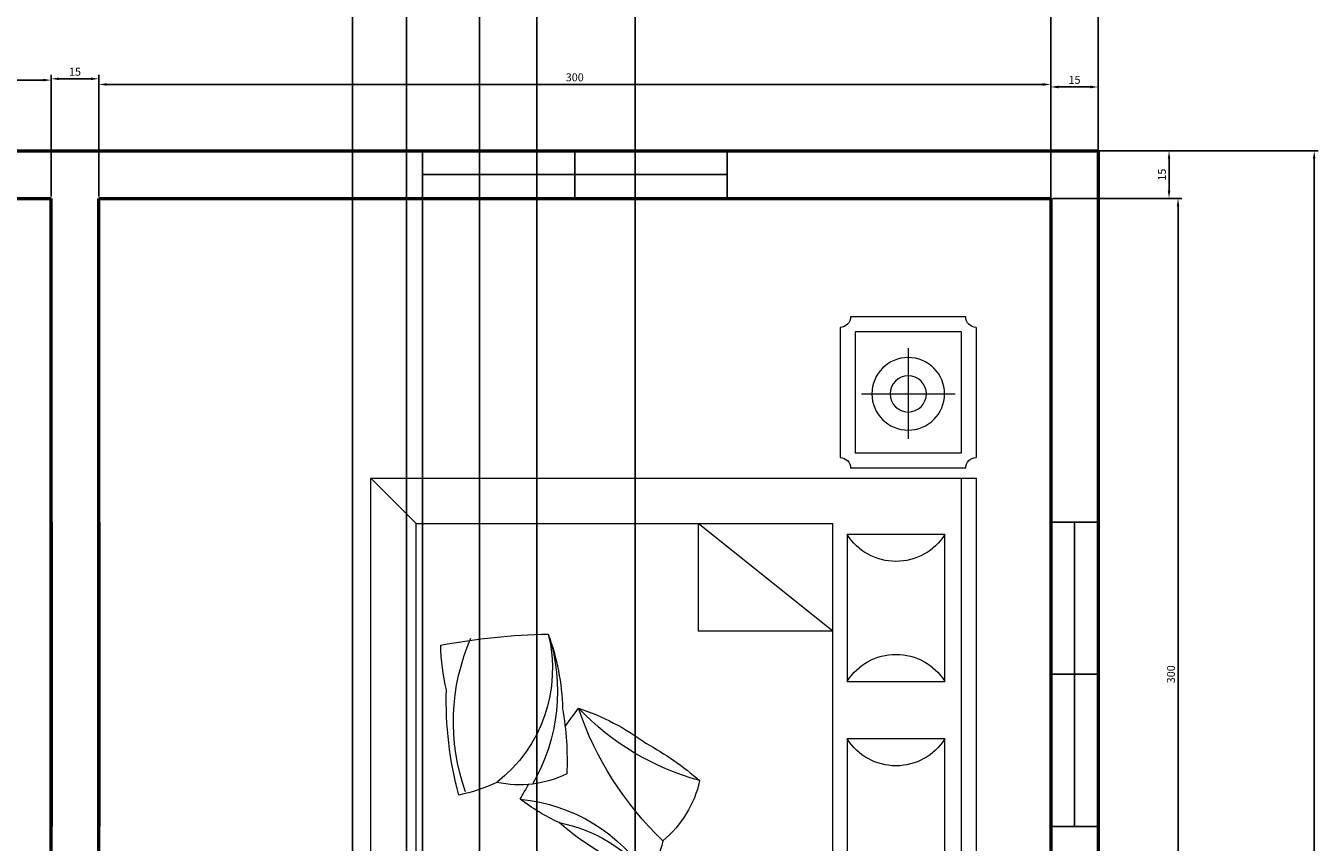
# Model space of a CAD drawing. Units: inches. Extents: x 604 to 3492, y -123 to 1737.
# Tile 17 of 20: x 1912 to 2319, y 1070 to 1327. Entities that reach past the tile are written whole.
import ezdxf

# ---------------------------------------------------------------- set-up
doc = ezdxf.new("R2010")
doc.units = ezdxf.units.IN
for name, color, linetype, lineweight in [('A-ANNO-DIMS', 2, 'Continuous', 18), ('A-FURN', 8, 'Continuous', 18), ('A-GLAZ', 4, 'Continuous', 25), ('A-WALL', 7, 'Continuous', 50)]:
    doc.layers.add(name, color=color, linetype=linetype, lineweight=lineweight)
doc.styles.get("Standard").update_dxf_attribs({"font": 'arial.ttf'})
doc.dimstyles.new('ISO-25', dxfattribs={"dimtxt": 2.5, "dimasz": 2.5, "dimexe": 1.25, "dimexo": 0.625, "dimtad": 1, "dimtxsty": 'Standard', "dimcen": 2.5, "dimadec": 0, "dimazin": 0, "dimtfac": 1, "dimtmove": 0, "dimatfit": 3, "dimfxl": 1, "dimarcsym": 0})

# ---------------------------------------------------------------- blocks, each defined once
blk = doc.blocks.new('A$C50B66110')
for p, q in [((0.0503, 1.9981), (0.4803, 1.9981)), ((0.1513, 1.6871), (0.1513, 1.9967)), ((0.5716, 1.9488), (0.5716, 2)), ((0.5716, 2), (2.0719, 2)), ((2.0719, 1.9488), (2.0719, 2)), ((2.1051, 1.9643), (2.1051, 1.5843)), ((2.5701, 1.9993), (2.1401, 1.9993)), ((2.6051, 1.9643), (2.6051, 1.5843)), ((0.0153, 1.9631), (0.0153, 1.5831)), ((0.0653, 1.9481), (0.0653, 1.5981)), ((0.0653, 1.9481), (0.4653, 1.9481)), ((0.4653, 1.9481), (0.4653, 1.5981)), ((0.5153, 1.9631), (0.5153, 1.5831)), ((2.0719, 1.9488), (0.5716, 1.9488)), ((0.5716, 1.9488), (0.5716, 0)), ((2.0719, 0), (2.0719, 1.9488)), ((2.1551, 1.9493), (2.1551, 1.5993)), ((2.5551, 1.9493), (2.1551, 1.9493)), ((2.3505, 1.62), (2.3505, 1.9295)), ((2.5551, 1.9493), (2.5551, 1.5993)), ((0.7257, 1.5725), (0.7257, 1.8954)), ((0.7257, 1.8954), (1.2113, 1.8954)), ((1.2113, 1.8954), (1.2113, 1.5725)), ((1.4007, 1.5725), (1.4007, 1.8954)), ((1.4007, 1.8954), (1.8863, 1.8954)), ((1.8863, 1.8954), (1.8863, 1.5725)), ((0, 1.8416), (0.2001, 1.8416)), ((2.5018, 1.7744), (2.2017, 1.7744)), ((0.0653, 1.5981), (0.4653, 1.5981)), ((2.5551, 1.5993), (2.1551, 1.5993)), ((0.0503, 1.5481), (0.4803, 1.5481)), ((1.2113, 1.5725), (0.7257, 1.5725)), ((1.8863, 1.5725), (1.4007, 1.5725)), ((2.5701, 1.5493), (2.1401, 1.5493)), ((1.5665, 1.5254), (1.5665, 1.0802)), ((1.5665, 1.5254), (1.9219, 1.0802)), ((1.9219, 1.0802), (1.5665, 1.0802)), ((0.5716, 0), (0.7216, 0.15)), ((2.0719, 0), (1.9219, 0.15)), ((0.5716, 0), (2.0719, 0))]:
    blk.add_line(p, q)
at = {"linetype": 'ByBlock'}
for p, q in [((0.2481, 1.9162), (0.2458, 1.9139)), ((0.2458, 1.9139), (0.2458, 1.7562)), ((0.2481, 1.9162), (0.4287, 1.9162)), ((0.2526, 1.9036), (0.2526, 1.8431)), ((0.3669, 1.9036), (0.2526, 1.9036)), ((0.3669, 1.8431), (0.3669, 1.9036)), ((0.3772, 1.9071), (0.3818, 1.9128)), ((0.3772, 1.7688), (0.3772, 1.9071)), ((0.3818, 1.9094), (0.3807, 1.9048)), ((0.3807, 1.9048), (0.3807, 1.8739)), ((0.3807, 1.9048), (0.3909, 1.8945)), ((0.3818, 1.9128), (0.4161, 1.9128)), ((0.3864, 1.9116), (0.3818, 1.9094)), ((0.3921, 1.8968), (0.3864, 1.9116)), ((0.3864, 1.9116), (0.4138, 1.9116)), ((0.3909, 1.8945), (0.3921, 1.8968)), ((0.3909, 1.8431), (0.3909, 1.8945)), ((0.4081, 1.8968), (0.3921, 1.8968)), ((0.4081, 1.8968), (0.4138, 1.9116)), ((0.4092, 1.8945), (0.4081, 1.8968)), ((0.4195, 1.9048), (0.4092, 1.8945)), ((0.4092, 1.8431), (0.4092, 1.8945)), ((0.4138, 1.9116), (0.4184, 1.9094)), ((0.4161, 1.9128), (0.4218, 1.9071)), ((0.4184, 1.9094), (0.4195, 1.9048)), ((0.4195, 1.9048), (0.4195, 1.8739)), ((0.4218, 1.9071), (0.4218, 1.7699)), ((0.4287, 1.9162), (0.4309, 1.9139)), ((0.4309, 1.9139), (0.4309, 1.7562)), ((0.2526, 1.8431), (0.3669, 1.8431)), ((0.2572, 1.8408), (0.2572, 1.8294)), ((0.3669, 1.8408), (0.2572, 1.8408)), ((0.2664, 1.8408), (0.2664, 1.8294)), ((0.2755, 1.8408), (0.2755, 1.8294)), ((0.2846, 1.8408), (0.2846, 1.8294)), ((0.2938, 1.8408), (0.2938, 1.8294)), ((0.3029, 1.8408), (0.3029, 1.8294)), ((0.3121, 1.8408), (0.3121, 1.8294)), ((0.3669, 1.8294), (0.3669, 1.8408)), ((0.3807, 1.8739), (0.3829, 1.8682)), ((0.3829, 1.8682), (0.3864, 1.8625)), ((0.3864, 1.8625), (0.3875, 1.8545)), ((0.3875, 1.8545), (0.3875, 1.8431)), ((0.3875, 1.8214), (0.3875, 1.8431)), ((0.3909, 1.8431), (0.3909, 1.7813)), ((0.4092, 1.8431), (0.4092, 1.7813)), ((0.4138, 1.8625), (0.4127, 1.8545)), ((0.4127, 1.8545), (0.4127, 1.8431)), ((0.4127, 1.8214), (0.4127, 1.8431)), ((0.4172, 1.8682), (0.4138, 1.8625)), ((0.4195, 1.8739), (0.4172, 1.8682)), ((0.3201, 1.8168), (0.2526, 1.8168)), ((0.2526, 1.8168), (0.2526, 1.7962)), ((0.2526, 1.7962), (0.3201, 1.7962)), ((0.2572, 1.8294), (0.3669, 1.8294)), ((0.2675, 1.8145), (0.2641, 1.8145)), ((0.2641, 1.8145), (0.2641, 1.8111)), ((0.2641, 1.8111), (0.2675, 1.8111)), ((0.2641, 1.8019), (0.2641, 1.7985)), ((0.2675, 1.8019), (0.2641, 1.8019)), ((0.2641, 1.7985), (0.2675, 1.7985)), ((0.2675, 1.8111), (0.2675, 1.8145)), ((0.2675, 1.7985), (0.2675, 1.8019)), ((0.2846, 1.8145), (0.2846, 1.8111)), ((0.2881, 1.8145), (0.2846, 1.8145)), ((0.2846, 1.8111), (0.2881, 1.8111)), ((0.2846, 1.8019), (0.2846, 1.7985)), ((0.2881, 1.8019), (0.2846, 1.8019)), ((0.2846, 1.7985), (0.2881, 1.7985)), ((0.2881, 1.8111), (0.2881, 1.8145)), ((0.2881, 1.7985), (0.2881, 1.8019)), ((0.3052, 1.8145), (0.3052, 1.8111)), ((0.3086, 1.8145), (0.3052, 1.8145)), ((0.3052, 1.8111), (0.3086, 1.8111)), ((0.3052, 1.8019), (0.3052, 1.7985)), ((0.3086, 1.8019), (0.3052, 1.8019)), ((0.3052, 1.7985), (0.3086, 1.7985)), ((0.3086, 1.8111), (0.3086, 1.8145)), ((0.3086, 1.7985), (0.3086, 1.8019)), ((0.3201, 1.7962), (0.3201, 1.8168)), ((0.3304, 1.8111), (0.3395, 1.8111)), ((0.3304, 1.8042), (0.3304, 1.8111)), ((0.3395, 1.8042), (0.3304, 1.8042)), ((0.3304, 1.7985), (0.3395, 1.7985)), ((0.3304, 1.7916), (0.3304, 1.7985)), ((0.3395, 1.8111), (0.3395, 1.8042)), ((0.3395, 1.7985), (0.3395, 1.7916)), ((0.3441, 1.8042), (0.3441, 1.8111)), ((0.3441, 1.8111), (0.3532, 1.8111)), ((0.3532, 1.8042), (0.3441, 1.8042)), ((0.3441, 1.7985), (0.3532, 1.7985)), ((0.3441, 1.7916), (0.3441, 1.7985)), ((0.3532, 1.8111), (0.3532, 1.8042)), ((0.3532, 1.7985), (0.3532, 1.7916)), ((0.3578, 1.8111), (0.3669, 1.8111)), ((0.3578, 1.8042), (0.3578, 1.8111)), ((0.3669, 1.8042), (0.3578, 1.8042)), ((0.3578, 1.7985), (0.3669, 1.7985)), ((0.3578, 1.7916), (0.3578, 1.7985)), ((0.3669, 1.8111), (0.3669, 1.8042)), ((0.3669, 1.7985), (0.3669, 1.7916)), ((0.3807, 1.8019), (0.3829, 1.8076)), ((0.3807, 1.7711), (0.3807, 1.8019)), ((0.3829, 1.8076), (0.3864, 1.8134)), ((0.3864, 1.8134), (0.3875, 1.8214)), ((0.4138, 1.8134), (0.4127, 1.8214)), ((0.4172, 1.8076), (0.4138, 1.8134)), ((0.4195, 1.8019), (0.4172, 1.8076)), ((0.4195, 1.7711), (0.4195, 1.8019)), ((0.2458, 1.7562), (0.2481, 1.7539)), ((0.4, 1.7539), (0.2481, 1.7539)), ((0.2652, 1.7905), (0.2538, 1.7905)), ((0.2538, 1.7905), (0.2538, 1.7859)), ((0.2538, 1.7859), (0.2652, 1.7859)), ((0.2538, 1.7665), (0.2538, 1.7733)), ((0.2538, 1.7733), (0.2652, 1.7733)), ((0.2652, 1.7665), (0.2538, 1.7665)), ((0.2652, 1.7859), (0.2652, 1.7905)), ((0.2652, 1.7733), (0.2652, 1.7665)), ((0.2812, 1.7905), (0.2698, 1.7905)), ((0.2698, 1.7905), (0.2698, 1.7859)), ((0.2698, 1.7859), (0.2812, 1.7859)), ((0.2698, 1.7665), (0.2698, 1.7733)), ((0.2698, 1.7733), (0.2812, 1.7733)), ((0.2812, 1.7665), (0.2698, 1.7665)), ((0.2812, 1.7859), (0.2812, 1.7905)), ((0.2812, 1.7733), (0.2812, 1.7665)), ((0.2972, 1.7905), (0.2858, 1.7905)), ((0.2858, 1.7905), (0.2858, 1.7859)), ((0.2858, 1.7859), (0.2972, 1.7859)), ((0.2858, 1.7665), (0.2858, 1.7733)), ((0.2858, 1.7733), (0.2972, 1.7733)), ((0.2972, 1.7665), (0.2858, 1.7665)), ((0.2972, 1.7859), (0.2972, 1.7905)), ((0.2972, 1.7733), (0.2972, 1.7665)), ((0.3018, 1.7905), (0.3018, 1.7859)), ((0.3132, 1.7905), (0.3018, 1.7905)), ((0.3018, 1.7859), (0.3132, 1.7859)), ((0.3018, 1.7733), (0.3132, 1.7733)), ((0.3018, 1.7665), (0.3018, 1.7733)), ((0.3132, 1.7665), (0.3018, 1.7665)), ((0.3132, 1.7859), (0.3132, 1.7905)), ((0.3132, 1.7733), (0.3132, 1.7665)), ((0.3395, 1.7916), (0.3304, 1.7916)), ((0.3304, 1.7779), (0.3304, 1.7848)), ((0.3304, 1.7848), (0.3395, 1.7848)), ((0.3395, 1.7779), (0.3304, 1.7779)), ((0.3304, 1.7722), (0.3395, 1.7722)), ((0.3304, 1.7653), (0.3304, 1.7722)), ((0.3395, 1.7653), (0.3304, 1.7653)), ((0.3395, 1.7848), (0.3395, 1.7779)), ((0.3395, 1.7722), (0.3395, 1.7653)), ((0.3532, 1.7916), (0.3441, 1.7916)), ((0.3441, 1.7779), (0.3441, 1.7848)), ((0.3441, 1.7848), (0.3532, 1.7848)), ((0.3532, 1.7779), (0.3441, 1.7779)), ((0.3441, 1.7722), (0.3532, 1.7722)), ((0.3441, 1.7653), (0.3441, 1.7722)), ((0.3532, 1.7653), (0.3441, 1.7653)), ((0.3532, 1.7848), (0.3532, 1.7779)), ((0.3532, 1.7722), (0.3532, 1.7653)), ((0.3669, 1.7916), (0.3578, 1.7916)), ((0.3578, 1.7791), (0.3578, 1.7859)), ((0.3578, 1.7859), (0.3669, 1.7859)), ((0.3669, 1.7791), (0.3578, 1.7791)), ((0.3578, 1.7653), (0.3578, 1.7722)), ((0.3578, 1.7722), (0.3669, 1.7722)), ((0.3669, 1.7653), (0.3578, 1.7653)), ((0.3669, 1.7859), (0.3669, 1.7791)), ((0.3669, 1.7722), (0.3669, 1.7653)), ((0.3829, 1.7631), (0.3772, 1.7688)), ((0.3807, 1.7711), (0.3909, 1.7813)), ((0.3818, 1.7665), (0.3807, 1.7711)), ((0.3864, 1.7642), (0.3818, 1.7665)), ((0.399, 1.7631), (0.3829, 1.7631)), ((0.3921, 1.7791), (0.3864, 1.7642)), ((0.3864, 1.7642), (0.399, 1.7642)), ((0.3909, 1.7813), (0.3921, 1.7791)), ((0.4081, 1.7791), (0.3921, 1.7791)), ((0.4024, 1.7676), (0.3989, 1.7676)), ((0.3989, 1.7676), (0.3991, 1.7578)), ((0.3991, 1.7578), (0.4019, 1.7462)), ((0.403, 1.7585), (0.4024, 1.7676)), ((0.4026, 1.7642), (0.4138, 1.7642)), ((0.4161, 1.7631), (0.4027, 1.7631)), ((0.4047, 1.7511), (0.403, 1.7585)), ((0.4287, 1.7539), (0.404, 1.7539)), ((0.4074, 1.7402), (0.4047, 1.7511)), ((0.4092, 1.7813), (0.4081, 1.7791)), ((0.4081, 1.7791), (0.4138, 1.7642)), ((0.4195, 1.7711), (0.4092, 1.7813)), ((0.4138, 1.7642), (0.4184, 1.7665)), ((0.4218, 1.7699), (0.4161, 1.7631)), ((0.4184, 1.7665), (0.4195, 1.7711)), ((0.4309, 1.7562), (0.4287, 1.7539)), ((0.4378, 1.7742), (0.4309, 1.7768)), ((0.4309, 1.7722), (0.436, 1.7708)), ((0.436, 1.7708), (0.4406, 1.7672)), ((0.441, 1.771), (0.4378, 1.7742)), ((0.4406, 1.7672), (0.4418, 1.7656)), ((0.4434, 1.7688), (0.441, 1.771)), ((0.4443, 1.7658), (0.4418, 1.7633)), ((0.4418, 1.7656), (0.4443, 1.7658)), ((0.4418, 1.7633), (0.4511, 1.7551)), ((0.4477, 1.7704), (0.4434, 1.7688)), ((0.4497, 1.7684), (0.4477, 1.7704)), ((0.4481, 1.765), (0.4497, 1.7684)), ((0.4509, 1.7672), (0.4481, 1.765)), ((0.4539, 1.764), (0.4509, 1.7672)), ((0.4511, 1.7551), (0.4662, 1.7422)), ((0.4515, 1.7573), (0.4539, 1.764)), ((0.4577, 1.7605), (0.4515, 1.7573)), ((0.463, 1.7555), (0.4577, 1.7605)), ((0.4618, 1.7482), (0.463, 1.7555)), ((0.467, 1.7515), (0.4618, 1.7482)), ((0.4714, 1.7468), (0.467, 1.7515)), ((0.4019, 1.7462), (0.4047, 1.7353)), ((0.4026, 1.7254), (0.4021, 1.7198)), ((0.4021, 1.7198), (0.4088, 1.7187)), ((0.4088, 1.7187), (0.4023, 1.7147)), ((0.4023, 1.7147), (0.4028, 1.7085)), ((0.4051, 1.7279), (0.4026, 1.7254)), ((0.4028, 1.7085), (0.4102, 1.7078)), ((0.4102, 1.7078), (0.4037, 1.7027)), ((0.4047, 1.7353), (0.4044, 1.7293)), ((0.4044, 1.7293), (0.4051, 1.7279)), ((0.4081, 1.7346), (0.4074, 1.7402)), ((0.4079, 1.7286), (0.4081, 1.7346)), ((0.4121, 1.7256), (0.4079, 1.7286)), ((0.4111, 1.7203), (0.4121, 1.7256)), ((0.4123, 1.7057), (0.4111, 1.7203)), ((0.4664, 1.7418), (0.4741, 1.72)), ((0.4696, 1.7418), (0.4714, 1.7468)), ((0.4766, 1.7425), (0.4697, 1.7418)), ((0.4741, 1.72), (0.4708, 1.7027)), ((0.472, 1.733), (0.4787, 1.7356)), ((0.4794, 1.7332), (0.472, 1.733)), ((0.4743, 1.7075), (0.4815, 1.7073)), ((0.4798, 1.7013), (0.4743, 1.7075)), ((0.4761, 1.7233), (0.481, 1.7279)), ((0.4824, 1.7233), (0.4761, 1.7233)), ((0.4764, 1.7154), (0.4835, 1.7175)), ((0.4824, 1.7119), (0.4764, 1.7154)), ((0.4787, 1.7356), (0.4766, 1.7425)), ((0.481, 1.7279), (0.4794, 1.7332)), ((0.4815, 1.7073), (0.4824, 1.7119)), ((0.4835, 1.7175), (0.4824, 1.7233)), ((0.4037, 1.7027), (0.4067, 1.6974)), ((0.4067, 1.6974), (0.4137, 1.6988)), ((0.4137, 1.6988), (0.4104, 1.6923)), ((0.4104, 1.6923), (0.4139, 1.6881)), ((0.4211, 1.6946), (0.4123, 1.7057)), ((0.4139, 1.6881), (0.4192, 1.692)), ((0.4192, 1.692), (0.4183, 1.6858)), ((0.4183, 1.6858), (0.4227, 1.683)), ((0.4333, 1.6881), (0.4211, 1.6946)), ((0.4227, 1.683), (0.4283, 1.6876)), ((0.4283, 1.6876), (0.4276, 1.68)), ((0.4276, 1.68), (0.4324, 1.6786)), ((0.4324, 1.6786), (0.4354, 1.6849)), ((0.4472, 1.6869), (0.4333, 1.6881)), ((0.4354, 1.6849), (0.4382, 1.6786)), ((0.4382, 1.6786), (0.4421, 1.6782)), ((0.4421, 1.6782), (0.4437, 1.6849)), ((0.4437, 1.6849), (0.4463, 1.6775)), ((0.4463, 1.6775), (0.4507, 1.6786)), ((0.4606, 1.6927), (0.4472, 1.6869)), ((0.4507, 1.6786), (0.4509, 1.6849)), ((0.4509, 1.6849), (0.4562, 1.6802)), ((0.4562, 1.6802), (0.4599, 1.6821)), ((0.4592, 1.689), (0.4641, 1.683)), ((0.4599, 1.6821), (0.4592, 1.689)), ((0.4708, 1.7027), (0.4606, 1.6927)), ((0.4641, 1.683), (0.4678, 1.6863)), ((0.465, 1.6925), (0.4715, 1.6897)), ((0.4678, 1.6863), (0.465, 1.6925)), ((0.4745, 1.6925), (0.4713, 1.6988)), ((0.4713, 1.6988), (0.478, 1.6967)), ((0.4715, 1.6897), (0.4745, 1.6925)), ((0.478, 1.6967), (0.4798, 1.7013)), ((0.7216, 1.5254), (1.9219, 1.5254)), ((0.7216, 1.5254), (0.7216, 0.15)), ((1.9219, 0.15), (1.9219, 1.5254)), ((0.7216, 0.15), (1.9219, 0.15))]:
    blk.add_line(p, q, dxfattribs=at)
for centre, radius in [((0.1513, 1.8416), 0.12), ((0.1513, 1.8416), 0.06), ((2.3505, 1.7744), 0.12), ((2.3505, 1.7744), 0.06)]:
    blk.add_circle(centre, radius)
for centre, radius, start, end in [((0.0153, 1.9981), 0.035, 270, 0), ((0.5153, 1.9981), 0.035, 180, 270), ((2.1051, 1.9993), 0.035, 270, 0), ((2.6051, 1.9993), 0.035, 180, 270), ((0.6244, 1.734), 0.1906, 302.1202, 57.8798), ((1.3126, 1.734), 0.1906, 122.1202, 237.8798), ((1.2994, 1.734), 0.1906, 302.1202, 57.8798), ((1.9876, 1.734), 0.1906, 122.1202, 237.8798), ((0.0153, 1.5481), 0.035, 0, 90), ((0.5153, 1.5481), 0.035, 90, 180), ((2.1051, 1.5493), 0.035, 0, 90), ((2.6051, 1.5493), 0.035, 90, 180), ((1.1502, 0.7366), 0.3575, 102.4782, 140.4625), ((0.328, 0.4368), 0.9879, 28.4971, 41.0566), ((1.9117, 1.3157), 0.8697, 195.336, 226.4193), ((0.9996, 0.4307), 0.548, 103.2034, 117.0362), ((1.656, 1.7093), 1.0798, 223.6306, 251.4288), ((0.4482, 0.4408), 0.5655, 5.3391, 57.6895), ((1.8226, 1.3753), 1.1652, 203.0642, 220.3209), ((0.4548, 0.5307), 0.4879, 10.6986, 52.6864), ((0.5648, 0.4378), 0.7874, 18.3527, 36.6851), ((-0.0179, 2.4352), 2.1977, 305.2966, 307.2418), ((1.4166, 0.4903), 0.3575, 154.0418, 192.0262), ((1.1403, -0.3401), 0.9879, 80.0607, 92.6202), ((1.5981, 0.9345), 0.734, 205.259, 216.9351), ((1.3672, 0.0075), 0.6085, 71.81, 120.1351), ((1.4431, 0.1219), 0.4774, 76.1849, 142.0017), ((1.2867, -0.154), 0.7874, 69.9163, 88.2487), ((-0.6401, 0.6314), 2.1977, 349.4884, 358.8054), ((-0.0179, 2.4352), 2.1977, 297.9248, 299.3793), ((1.5626, 0.1822), 0.548, 154.767, 168.5998), ((1.2678, 0.9611), 0.6885, 250.2936, 293.6414), ((1.3343, 1.4141), 1.1652, 254.6278, 271.8845), ((1.5399, 0.9642), 0.734, 256.8226, 268.4988)]:
    blk.add_arc(centre, radius, start, end)
blk = doc.blocks.new('*D39')
at = {"layer": 'A-ANNO-DIMS', "color": 0, "lineweight": -2, "transparency": 16777216}
for p, q in [((1589.57, 1273.33), (1589.57, 1311.26)), ((1592.07, 1310.01), (1917.07, 1310.01)), ((1919.57, 1273.33), (1919.57, 1311.26))]:
    blk.add_line(p, q, dxfattribs=at)
at = {"layer": 'A-ANNO-DIMS', "color": 0, "transparency": 16777216}
for points in [[(1592.07, 1310.43), (1592.07, 1309.59), (1589.57, 1310.01)], [(1917.07, 1310.43), (1917.07, 1309.59), (1919.57, 1310.01)]]:
    blk.add_solid(points, dxfattribs=at)
at = {"layer": 'Defpoints', "color": 0, "transparency": 16777216}
for p in [(1919.57, 1310.01), (1589.57, 1272.7), (1919.57, 1272.7)]:
    blk.add_point(p, dxfattribs=at)
at = {"layer": 'A-ANNO-DIMS', "color": 0, "transparency": 16777216, "insert": (1754.57, 1311.91), "char_height": 2.5, "attachment_point": 5}
blk.add_mtext('330', dxfattribs=at)
blk = doc.blocks.new('*D40')
at = {"layer": 'A-ANNO-DIMS', "color": 0, "lineweight": -2, "transparency": 16777216}
for p, q in [((1919.57, 1273.33), (1919.57, 1311.67)), ((1934.57, 1273.33), (1934.57, 1311.67)), ((1922.07, 1310.42), (1932.07, 1310.42))]:
    blk.add_line(p, q, dxfattribs=at)
at = {"layer": 'A-ANNO-DIMS', "color": 0, "transparency": 16777216}
for points in [[(1922.07, 1310.84), (1922.07, 1310), (1919.57, 1310.42)], [(1932.07, 1310.84), (1932.07, 1310), (1934.57, 1310.42)]]:
    blk.add_solid(points, dxfattribs=at)
at = {"layer": 'Defpoints', "color": 0, "transparency": 16777216}
for p in [(1934.57, 1310.42), (1919.57, 1272.7), (1934.57, 1272.7)]:
    blk.add_point(p, dxfattribs=at)
at = {"layer": 'A-ANNO-DIMS', "color": 0, "transparency": 16777216, "insert": (1927.07, 1312.32), "char_height": 2.5, "attachment_point": 5}
blk.add_mtext('15', dxfattribs=at)
blk = doc.blocks.new('*D41')
at = {"layer": 'A-ANNO-DIMS', "color": 0, "lineweight": -2, "transparency": 16777216}
for p, q in [((1934.57, 1273.33), (1934.57, 1309.89)), ((1937.07, 1308.64), (2232.07, 1308.64)), ((2234.57, 1273.33), (2234.57, 1309.89))]:
    blk.add_line(p, q, dxfattribs=at)
at = {"layer": 'A-ANNO-DIMS', "color": 0, "transparency": 16777216}
for points in [[(1937.07, 1309.06), (1937.07, 1308.23), (1934.57, 1308.64)], [(2232.07, 1309.06), (2232.07, 1308.23), (2234.57, 1308.64)]]:
    blk.add_solid(points, dxfattribs=at)
at = {"layer": 'Defpoints', "color": 0, "transparency": 16777216}
for p in [(2234.57, 1308.64), (1934.57, 1272.7), (2234.57, 1272.7)]:
    blk.add_point(p, dxfattribs=at)
at = {"layer": 'A-ANNO-DIMS', "color": 0, "transparency": 16777216, "insert": (2084.57, 1310.55), "char_height": 2.5, "attachment_point": 5}
blk.add_mtext('300', dxfattribs=at)
blk = doc.blocks.new('*D42')
at = {"layer": 'A-ANNO-DIMS', "color": 0, "lineweight": -2, "transparency": 16777216}
for p, q in [((2234.57, 1273.33), (2234.57, 1309.09)), ((2237.07, 1307.84), (2247.07, 1307.84)), ((2249.57, 1273.33), (2249.57, 1309.09))]:
    blk.add_line(p, q, dxfattribs=at)
at = {"layer": 'A-ANNO-DIMS', "color": 0, "transparency": 16777216}
for points in [[(2237.07, 1308.26), (2237.07, 1307.42), (2234.57, 1307.84)], [(2247.07, 1308.26), (2247.07, 1307.42), (2249.57, 1307.84)]]:
    blk.add_solid(points, dxfattribs=at)
at = {"layer": 'Defpoints', "color": 0, "transparency": 16777216}
for p in [(2249.57, 1307.84), (2234.57, 1272.7), (2249.57, 1272.7)]:
    blk.add_point(p, dxfattribs=at)
at = {"layer": 'A-ANNO-DIMS', "color": 0, "transparency": 16777216, "insert": (2242.07, 1309.74), "char_height": 2.5, "attachment_point": 5}
blk.add_mtext('15', dxfattribs=at)
blk = doc.blocks.new('*D43')
at = {"layer": 'A-ANNO-DIMS', "color": 0, "lineweight": -2, "transparency": 16777216}
for p, q in [((2235.2, 1287.7), (2273.12, 1287.7)), ((2271.87, 1285.2), (2271.87, 1275.2)), ((2235.2, 1272.7), (2273.12, 1272.7))]:
    blk.add_line(p, q, dxfattribs=at)
at = {"layer": 'A-ANNO-DIMS', "color": 0, "transparency": 16777216}
for points in [[(2271.46, 1285.2), (2272.29, 1285.2), (2271.87, 1287.7)], [(2271.46, 1275.2), (2272.29, 1275.2), (2271.87, 1272.7)]]:
    blk.add_solid(points, dxfattribs=at)
at = {"layer": 'Defpoints', "color": 0, "transparency": 16777216}
for p in [(2234.57, 1287.7), (2234.57, 1272.7), (2271.87, 1272.7)]:
    blk.add_point(p, dxfattribs=at)
at = {"layer": 'A-ANNO-DIMS', "color": 0, "transparency": 16777216, "insert": (2269.97, 1280.2), "char_height": 2.5, "attachment_point": 5, "rotation": 90}
blk.add_mtext('15', dxfattribs=at)
blk = doc.blocks.new('*D44')
at = {"layer": 'A-ANNO-DIMS', "color": 0, "lineweight": -2, "transparency": 16777216}
for p, q in [((2235.2, 1272.7), (2275.95, 1272.7)), ((2274.7, 975.2), (2274.7, 1270.2)), ((2235.2, 972.7), (2275.95, 972.7))]:
    blk.add_line(p, q, dxfattribs=at)
at = {"layer": 'A-ANNO-DIMS', "color": 0, "transparency": 16777216}
for points in [[(2274.28, 1270.2), (2275.11, 1270.2), (2274.7, 1272.7)], [(2274.28, 975.2), (2275.11, 975.2), (2274.7, 972.7)]]:
    blk.add_solid(points, dxfattribs=at)
at = {"layer": 'Defpoints', "color": 0, "transparency": 16777216}
for p in [(2234.57, 1272.7), (2274.7, 1272.7), (2234.57, 972.7)]:
    blk.add_point(p, dxfattribs=at)
at = {"layer": 'A-ANNO-DIMS', "color": 0, "transparency": 16777216, "insert": (2272.79, 1122.7), "char_height": 2.5, "attachment_point": 5, "rotation": 90}
blk.add_mtext('300', dxfattribs=at)
blk = doc.blocks.new('*D70')
at = {"layer": 'A-ANNO-DIMS', "color": 0, "lineweight": -2, "transparency": 16777216}
for p, q in [((2250.2, 1287.7), (2318.86, 1287.7)), ((2317.61, 455.2), (2317.61, 1285.2)), ((2250.2, 452.7), (2318.86, 452.7))]:
    blk.add_line(p, q, dxfattribs=at)
at = {"layer": 'A-ANNO-DIMS', "color": 0, "transparency": 16777216}
for points in [[(2317.2, 1285.2), (2318.03, 1285.2), (2317.61, 1287.7)], [(2317.2, 455.2), (2318.03, 455.2), (2317.61, 452.7)]]:
    blk.add_solid(points, dxfattribs=at)
at = {"layer": 'Defpoints', "color": 0, "transparency": 16777216}
for p in [(2249.57, 1287.7), (2317.61, 1287.7), (2249.57, 452.7)]:
    blk.add_point(p, dxfattribs=at)
at = {"layer": 'A-ANNO-DIMS', "color": 0, "transparency": 16777216, "insert": (2315.71, 870.2), "char_height": 2.5, "attachment_point": 5, "rotation": 90}
blk.add_mtext('835', dxfattribs=at)
blk = doc.blocks.new('*D71')
at = {"layer": 'A-ANNO-DIMS', "color": 0, "lineweight": -2, "transparency": 16777216}
for p, q in [((1574.57, 1288.33), (1574.57, 1357.82)), ((1577.07, 1356.57), (2247.07, 1356.57)), ((2249.57, 1288.33), (2249.57, 1357.82))]:
    blk.add_line(p, q, dxfattribs=at)
at = {"layer": 'A-ANNO-DIMS', "color": 0, "transparency": 16777216}
for points in [[(1577.07, 1356.98), (1577.07, 1356.15), (1574.57, 1356.57)], [(2247.07, 1356.98), (2247.07, 1356.15), (2249.57, 1356.57)]]:
    blk.add_solid(points, dxfattribs=at)
at = {"layer": 'Defpoints', "color": 0, "transparency": 16777216}
for p in [(2249.57, 1356.57), (1574.57, 1287.7), (2249.57, 1287.7)]:
    blk.add_point(p, dxfattribs=at)
at = {"layer": 'A-ANNO-DIMS', "color": 0, "transparency": 16777216, "insert": (1912.07, 1358.47), "char_height": 2.5, "attachment_point": 5}
blk.add_mtext('675', dxfattribs=at)
blk = doc.blocks.new('WIN-96')
for p, q in [((15, 96), (0, 96)), ((7.5, 96), (7.5, 0)), ((15, 96), (15, 0)), ((15, 48), (0, 48))]:
    blk.add_line(p, q)
blk.add_lwpolyline([(0, 96), (0, 0), (15, 0), (15, 96)], close=True)
blk = doc.blocks.new('*D101')
at = {"layer": 'A-ANNO-DIMS', "color": 0, "lineweight": -2, "transparency": 16777216}
for p, q in [((2031.57, 843.33), (2031.57, 1359.9)), ((2034.07, 1358.65), (2232.07, 1358.65)), ((2234.57, 843.33), (2234.57, 1359.9))]:
    blk.add_line(p, q, dxfattribs=at)
at = {"layer": 'A-ANNO-DIMS', "color": 0, "transparency": 16777216}
for points in [[(2034.07, 1359.07), (2034.07, 1358.23), (2031.57, 1358.65)], [(2232.07, 1359.07), (2232.07, 1358.23), (2234.57, 1358.65)]]:
    blk.add_solid(points, dxfattribs=at)
at = {"layer": 'Defpoints', "color": 0, "transparency": 16777216}
for p in [(2234.57, 1358.65), (2031.57, 842.7), (2234.57, 842.7)]:
    blk.add_point(p, dxfattribs=at)
at = {"layer": 'A-ANNO-DIMS', "color": 0, "transparency": 16777216, "insert": (2133.07, 1360.55), "char_height": 2.5, "attachment_point": 5}
blk.add_mtext('203', dxfattribs=at)
blk = doc.blocks.new('*D104')
at = {"layer": 'A-ANNO-DIMS', "color": 0, "lineweight": -2, "transparency": 16777216}
for p, q in [((1934.57, 1272.08), (1934.57, 215.5)), ((2036.57, 1272.08), (2036.57, 215.5)), ((1937.07, 216.75), (2034.07, 216.75))]:
    blk.add_line(p, q, dxfattribs=at)
at = {"layer": 'A-ANNO-DIMS', "color": 0, "transparency": 16777216}
for points in [[(1937.07, 217.17), (1937.07, 216.33), (1934.57, 216.75)], [(2034.07, 217.17), (2034.07, 216.33), (2036.57, 216.75)]]:
    blk.add_solid(points, dxfattribs=at)
at = {"layer": 'Defpoints', "color": 0, "transparency": 16777216}
for p in [(1934.57, 1272.7), (2036.57, 1272.7), (2036.57, 216.75)]:
    blk.add_point(p, dxfattribs=at)
at = {"layer": 'A-ANNO-DIMS', "color": 0, "transparency": 16777216, "insert": (1985.57, 218.65), "char_height": 2.5, "attachment_point": 5}
blk.add_mtext('102', dxfattribs=at)
blk = doc.blocks.new('*D109')
at = {"layer": 'A-ANNO-DIMS', "color": 0, "lineweight": -2, "transparency": 16777216}
for p, q in [((2054.57, 740.33), (2054.57, 1359.9)), ((2057.07, 1358.65), (2232.07, 1358.65)), ((2234.57, 740.33), (2234.57, 1359.9))]:
    blk.add_line(p, q, dxfattribs=at)
at = {"layer": 'A-ANNO-DIMS', "color": 0, "transparency": 16777216}
for points in [[(2057.07, 1359.07), (2057.07, 1358.23), (2054.57, 1358.65)], [(2232.07, 1359.07), (2232.07, 1358.23), (2234.57, 1358.65)]]:
    blk.add_solid(points, dxfattribs=at)
at = {"layer": 'Defpoints', "color": 0, "transparency": 16777216}
for p in [(2234.57, 1358.65), (2054.57, 739.7), (2234.57, 739.7)]:
    blk.add_point(p, dxfattribs=at)
at = {"layer": 'A-ANNO-DIMS', "color": 0, "transparency": 16777216, "insert": (2144.57, 1360.55), "char_height": 2.5, "attachment_point": 5}
blk.add_mtext('180', dxfattribs=at)
blk = doc.blocks.new('*D111')
at = {"layer": 'A-ANNO-DIMS', "color": 0, "lineweight": -2, "transparency": 16777216}
for p, q in [((2103.57, 973.33), (2103.57, 1359.9)), ((2106.07, 1358.65), (2232.07, 1358.65)), ((2234.57, 973.33), (2234.57, 1359.9))]:
    blk.add_line(p, q, dxfattribs=at)
at = {"layer": 'A-ANNO-DIMS', "color": 0, "transparency": 16777216}
for points in [[(2106.07, 1359.07), (2106.07, 1358.23), (2103.57, 1358.65)], [(2232.07, 1359.07), (2232.07, 1358.23), (2234.57, 1358.65)]]:
    blk.add_solid(points, dxfattribs=at)
at = {"layer": 'Defpoints', "color": 0, "transparency": 16777216}
for p in [(2234.57, 1358.65), (2103.57, 972.7), (2234.57, 972.7)]:
    blk.add_point(p, dxfattribs=at)
at = {"layer": 'A-ANNO-DIMS', "color": 0, "transparency": 16777216, "insert": (2169.07, 1360.55), "char_height": 2.5, "attachment_point": 5}
blk.add_mtext('131', dxfattribs=at)
blk = doc.blocks.new('*D113')
at = {"layer": 'A-ANNO-DIMS', "color": 0, "lineweight": -2, "transparency": 16777216}
for p, q in [((2014.57, 603.33), (2014.57, 1359.9)), ((2017.07, 1358.65), (2070.07, 1358.65)), ((2072.57, 603.33), (2072.57, 1359.9))]:
    blk.add_line(p, q, dxfattribs=at)
at = {"layer": 'A-ANNO-DIMS', "color": 0, "transparency": 16777216}
for points in [[(2017.07, 1359.07), (2017.07, 1358.23), (2014.57, 1358.65)], [(2070.07, 1359.07), (2070.07, 1358.23), (2072.57, 1358.65)]]:
    blk.add_solid(points, dxfattribs=at)
at = {"layer": 'Defpoints', "color": 0, "transparency": 16777216}
for p in [(2072.57, 1358.65), (2014.57, 602.7), (2072.57, 602.7)]:
    blk.add_point(p, dxfattribs=at)
at = {"layer": 'A-ANNO-DIMS', "color": 0, "transparency": 16777216, "insert": (2043.57, 1360.55), "char_height": 2.5, "attachment_point": 5}
blk.add_mtext('58', dxfattribs=at)

msp = doc.modelspace()

# ---------------------------------------------------------------- linework, layer by layer
at = {"layer": 'A-WALL'}
for p, q in [((1574.5743, 1287.7004), (2249.5743, 1287.7004)), ((2249.5743, 1287.7004), (2249.5743, 452.7004)), ((1589.5743, 1272.7004), (1919.5743, 1272.7004)), ((1589.5743, 1272.7004), (1919.5743, 1272.7004)), ((1919.5743, 972.7004), (1919.5743, 1272.7004)), ((1934.5743, 972.7004), (1934.5743, 1272.7004)), ((1934.5743, 1272.7004), (2234.5743, 1272.7004)), ((1934.5743, 972.7004), (1934.5743, 1272.7004)), ((1934.5743, 1272.7004), (2234.5743, 1272.7004)), ((2234.5743, 1272.7004), (2234.5743, 972.7004)), ((2234.5743, 1272.7004), (2234.5743, 972.7004)), ((1934.5743, 1170.7004), (1934.5743, 1074.7004))]:
    msp.add_line(p, q, dxfattribs=at)
for points in [[(1919.5743, 1170.7004), (1919.5743, 1074.7004)], [(1934.5743, 1074.7004), (1934.5743, 1170.7004)]]:
    msp.add_lwpolyline(points, dxfattribs=at)

# ---------------------------------------------------------------- block references
at = {"layer": 'A-FURN', "xscale": -95.4379570199766, "yscale": 95.4379570199766, "zscale": 95.4379570199766, "rotation": 270}
msp.add_blockref('A$C50B66110', (2020.3248, 986.7784), dxfattribs=at)
at = {"layer": 'A-GLAZ', "rotation": 89.99999999999905}
msp.add_blockref('WIN-96', (2132.5743, 1272.7004), dxfattribs=at)
at = {"layer": 'A-GLAZ'}
msp.add_blockref('WIN-96', (2234.5743, 1074.7004), dxfattribs=at)

# ---------------------------------------------------------------- dimensions: what is measured, and where the dimension line sits
at = {"layer": 'A-ANNO-DIMS'}
for base, p1, p2, override, picture, middle in [((2072.5743, 1358.6504), (2014.5743, 602.7004), (2072.5743, 602.7004), {"dimdec": 0, "dimlfac": 1, "dimrnd": 0, "dimzin": 0, "dimdsep": 46, "dimlunit": 2}, '*D113', (2043.5743, 1360.5519)), ((2234.5743, 1358.6504), (2031.5743, 842.7004), (2234.5743, 842.7004), {"dimdec": 0, "dimlfac": 1, "dimrnd": 0, "dimzin": 0, "dimdsep": 46, "dimlunit": 2}, '*D101', (2133.0743, 1360.5527)), ((2234.5743, 1358.6504), (2054.5743, 739.7004), (2234.5743, 739.7004), {"dimdec": 0, "dimlfac": 1, "dimrnd": 0, "dimzin": 0, "dimdsep": 46, "dimlunit": 2}, '*D109', (2144.5743, 1360.5519)), ((2234.5743, 1358.6504), (2103.5743, 972.7004), (2234.5743, 972.7004), {"dimdec": 0, "dimlfac": 1, "dimrnd": 0, "dimzin": 0, "dimdsep": 46, "dimlunit": 2}, '*D111', (2169.0743, 1360.5527)), ((1919.5743, 1310.0107), (1589.5743, 1272.7004), (1919.5743, 1272.7004), {"dimclrd": 0, "dimclre": 0, "dimclrt": 0}, '*D39', (1754.5743, 1311.913)), ((1934.5743, 1310.4212), (1919.5743, 1272.7004), (1934.5743, 1272.7004), {"dimclrd": 0, "dimclre": 0, "dimclrt": 0}, '*D40', (1927.0743, 1312.3226)), ((2234.5743, 1308.6428), (1934.5743, 1272.7004), (2234.5743, 1272.7004), {"dimclrd": 0, "dimclre": 0, "dimclrt": 0}, '*D41', (2084.5743, 1310.545)), ((2249.5743, 1307.8401), (2234.5743, 1272.7004), (2249.5743, 1272.7004), {"dimclrd": 0, "dimclre": 0, "dimclrt": 0}, '*D42', (2242.0743, 1309.7416)), ((2036.5743, 216.7504), (1934.5743, 1272.7004), (2036.5743, 1272.7004), {"dimdec": 0, "dimlfac": 1, "dimrnd": 0, "dimzin": 0, "dimdsep": 46, "dimlunit": 2}, '*D104', (1985.5743, 218.6519))]:
    dim = msp.add_linear_dim(base=base, p1=p1, p2=p2, dimstyle='ISO-25', override=override, dxfattribs=at)
    dim.commit()
    dim.dimension.update_dxf_attribs({"geometry": picture, "text_midpoint": middle})
for p1, distance, picture, middle in [((1574.5743, 1287.7004), 68.8648, '*D71', (1912.0743, 1358.4667)), ((2249.5743, 452.7004), -68.0392, '*D70', (2315.7113, 870.2004))]:
    dim = msp.add_aligned_dim(p1=p1, p2=(2249.5743, 1287.7004), distance=distance, dimstyle='ISO-25', override={"dimclrd": 0, "dimclre": 0, "dimclrt": 0}, dxfattribs=at)
    dim.commit()
    dim.dimension.update_dxf_attribs({"geometry": picture, "text_midpoint": middle})
for base, p1, picture, middle in [((2271.8739, 1272.7004), (2234.5743, 1287.7004), '*D43', (2269.9725, 1280.2004)), ((2274.6954, 1272.7004), (2234.5743, 972.7004), '*D44', (2272.7931, 1122.7004))]:
    dim = msp.add_linear_dim(base=base, p1=p1, p2=(2234.5743, 1272.7004), angle=90, dimstyle='ISO-25', override={"dimclrd": 0, "dimclre": 0, "dimclrt": 0}, dxfattribs=at)
    dim.commit()
    dim.dimension.update_dxf_attribs({"geometry": picture, "text_midpoint": middle})

doc.saveas('drawing.dxf')
